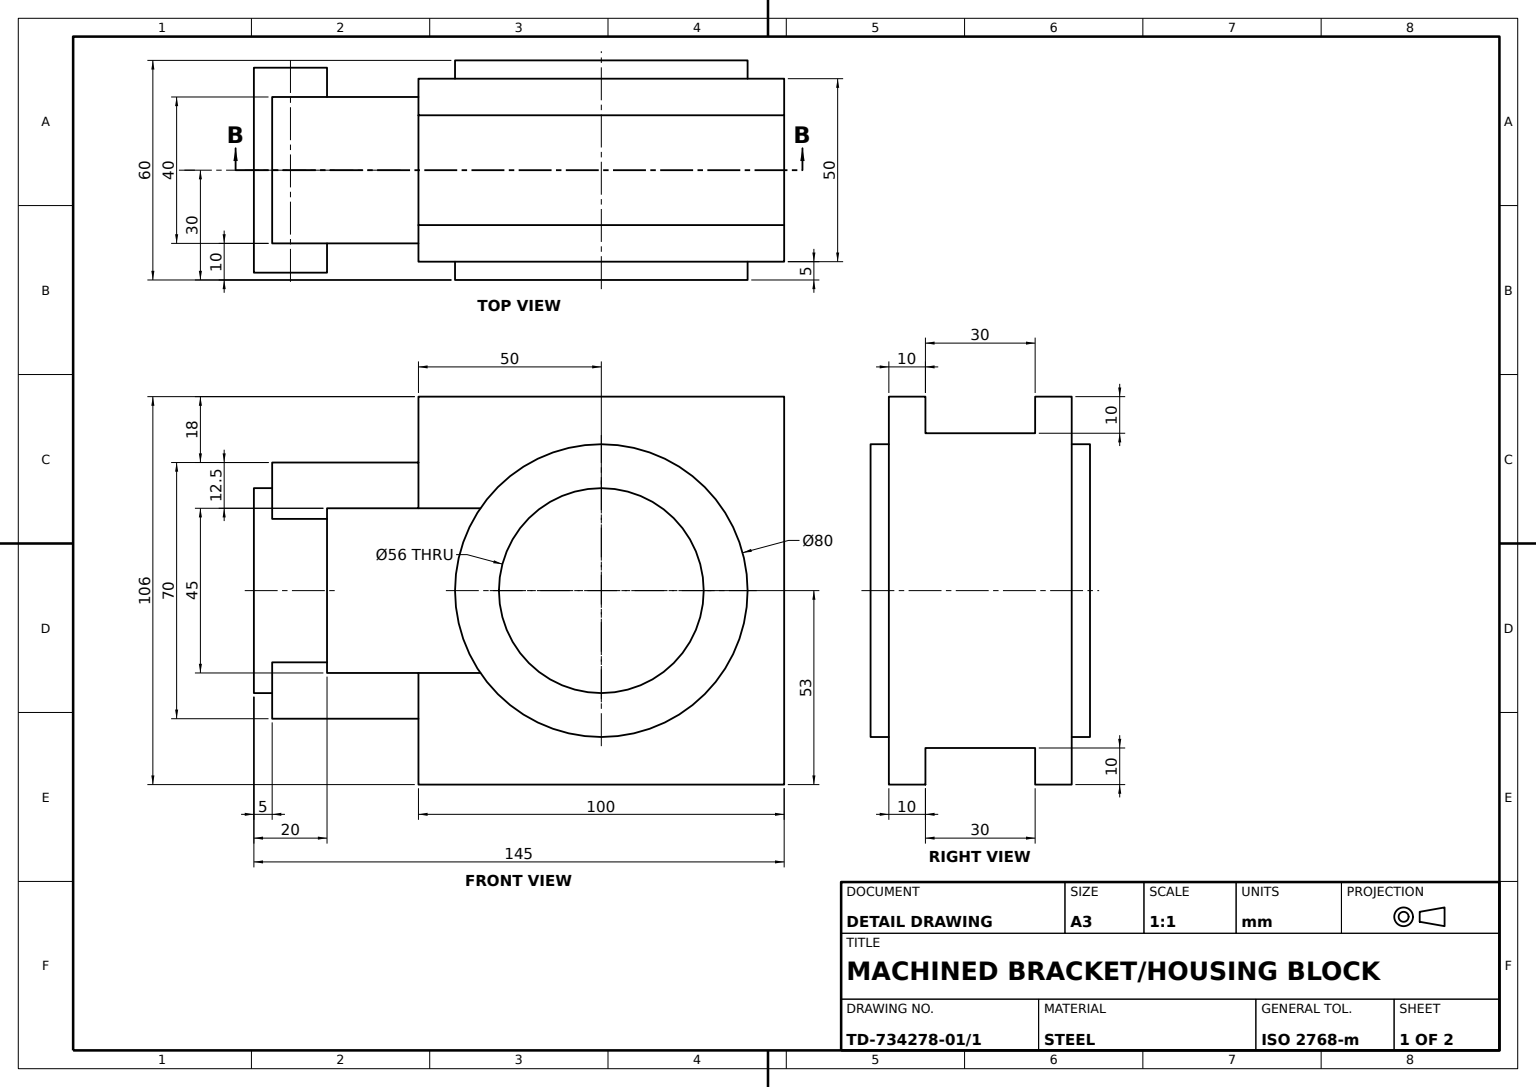
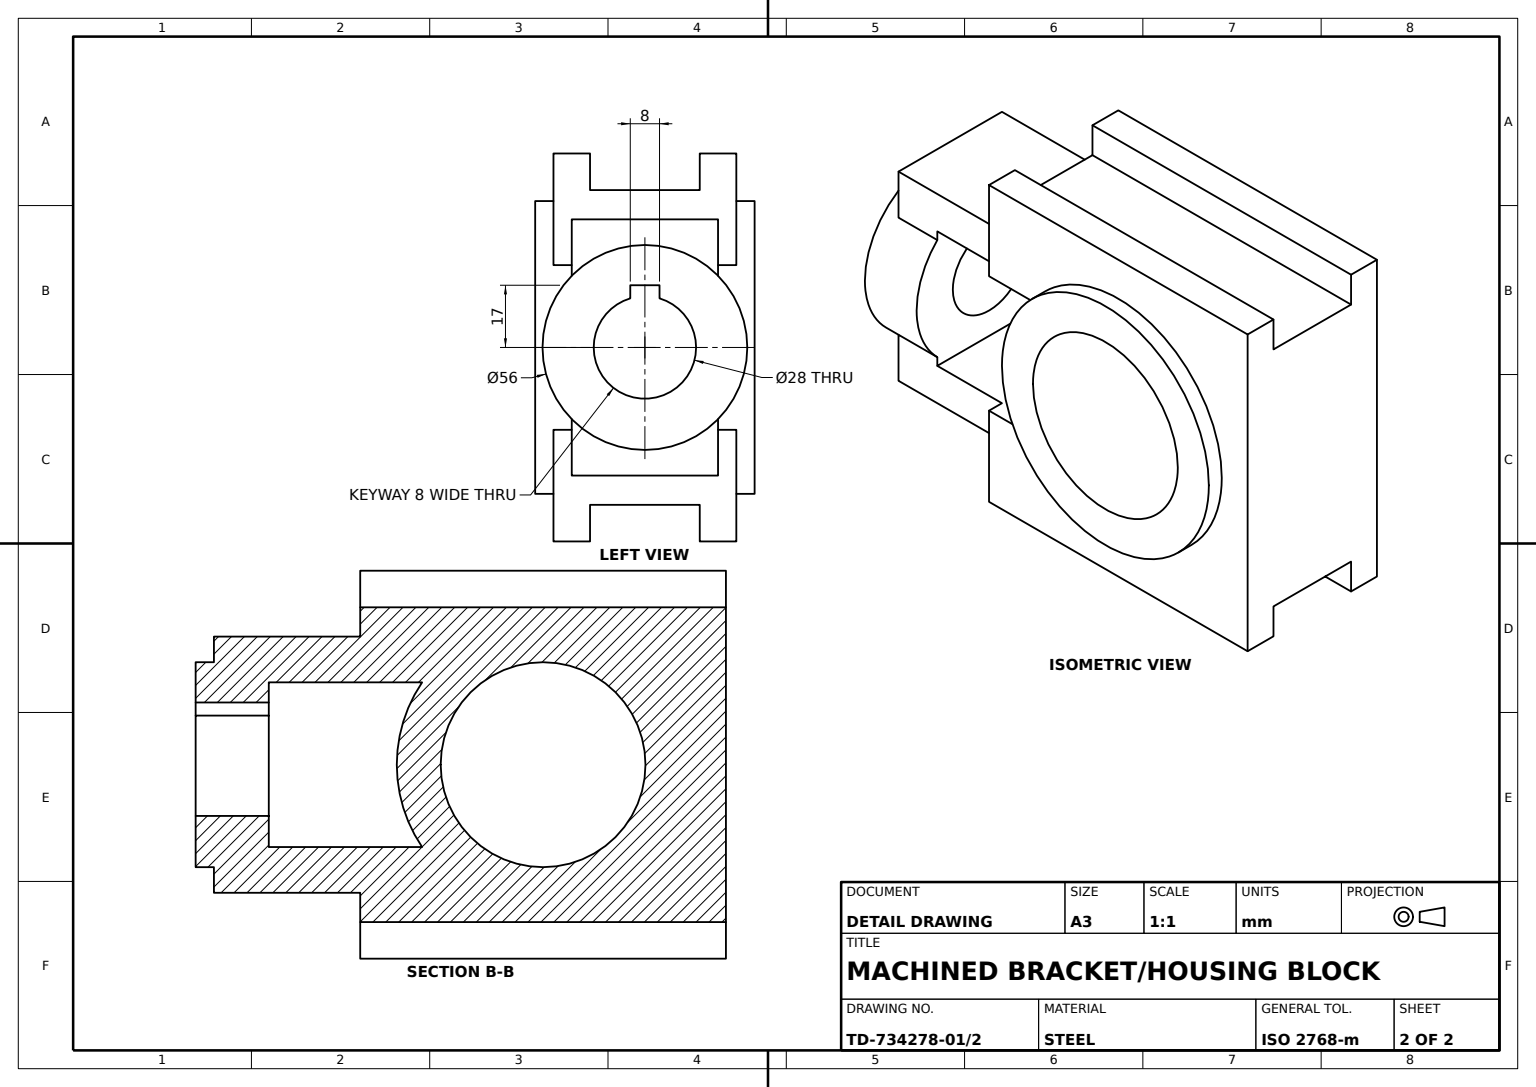
from build123d import *

# Parameters (mm, degrees)
BASE_BLOCK_DEPTH          = 50
BODY_RECESS_CUT_DEPTH     = 50
BEARING_HUB_PROFILE_R     = 40
BEARING_HUB_BOSS_DEPTH    = 50
HUB_START                 = 5
HUB_FLANGE_PROFILE_R      = 40
HUB_FLANGE_BOSS_DEPTH     = 5
MAIN_BORE_PROFILE_R       = 28
MAIN_BORE_CUT_DEPTH       = 113
TOP_SLOT_PROFILE_W        = 30
TOP_SLOT_PROFILE_H        = 100
TOP_SLOT_CUT_DEPTH        = 10
SIDE_ARM_BOSS_DEPTH       = 40
ARM_HOLE_PROFILE_R        = 28
ARM_HOLE_CUT_DEPTH        = 15
SHAFT_HUB_BOSS_DEPTH      = 5
SHAFT_HUB_BOSS_DEPTH_BACK = 15
SHAFT_HUB_PROFILE_R       = 28
KEYED_BORE_CUT_DEPTH      = 30
REAR_RING_PROFILE_R       = 40
REAR_RING_BOSS_DEPTH      = 5
THROUGH_BORE_PROFILE_R    = 28
THROUGH_BORE_CUT_DEPTH    = 194
SECOND_SLOT_PROFILE_W     = 30
SECOND_SLOT_PROFILE_H     = 100
SECOND_SLOT_CUT_DEPTH     = 10


with BuildPart() as part:
    # Base Block Profile → Base Block (new body)
    with BuildSketch(Plane(origin=(0, 0, 0), x_dir=(0, 0, -1), z_dir=(1, 0, 0))):
        Polygon((50, 0), (50, 53), (-50, 53), (-50, -53), (50, -53), align=None)
    extrude(amount=-BASE_BLOCK_DEPTH)

    # Body Recess Profile → Body Recess Cut (cut)
    with BuildSketch(Plane(origin=(0, 0, 0), x_dir=(0, 0, -1), z_dir=(1, 0, 0))):
        with BuildLine():
            Line((-50, 0), (-50, 22.5))
            Line((-50, 22.5), (-33.071891388, 22.5))
            ThreePointArc((-33.071891388, 22.5), (40, 0), (-33.071891388, -22.5))
            Line((-33.071891388, -22.5), (-50, -22.5))
            Line((-50, -22.5), (-50, 0))
        make_face()
    extrude(amount=-BODY_RECESS_CUT_DEPTH, mode=Mode.SUBTRACT)

    # Bearing Hub Profile → Bearing Hub Boss (add)
    with BuildSketch(Plane(origin=(0, 0, 0), x_dir=(0, 0, -1), z_dir=(1, 0, 0))):
        Circle(BEARING_HUB_PROFILE_R)
    extrude(amount=-BEARING_HUB_BOSS_DEPTH)

    # Hub Flange Profile → Hub Flange Boss (add)
    with BuildSketch(Plane(origin=(0, 0, 0), x_dir=(0, 0, -1), z_dir=(1, 0, 0)).offset(HUB_START)):
        Circle(HUB_FLANGE_PROFILE_R)
    extrude(amount=-HUB_FLANGE_BOSS_DEPTH)

    # Main Bore Profile → Main Bore Cut (cut)
    with BuildSketch(Plane(origin=(5, 0, 0), x_dir=(0, 0, -1), z_dir=(1, 0, 0))):
        Circle(MAIN_BORE_PROFILE_R)
    extrude(amount=-MAIN_BORE_CUT_DEPTH, mode=Mode.SUBTRACT)

    # Top Slot Profile → Top Slot Cut (cut)
    with BuildSketch(Plane(origin=(0, 53, 0), x_dir=(1, 0, 0), z_dir=(0, 1, 0))):
        with Locations((-25, 0)):
            Rectangle(TOP_SLOT_PROFILE_W, TOP_SLOT_PROFILE_H)
    extrude(amount=-TOP_SLOT_CUT_DEPTH, mode=Mode.SUBTRACT)

    # Side Arm Profile → Side Arm Boss (add)
    with BuildSketch(Plane(origin=(-5, 0, 0), x_dir=(0, 0, -1), z_dir=(1, 0, 0))):
        Polygon((-90, 0), (-90, 35), (-50, 35), (-50, 22.5), (-75, 22.5), (-75, -22.5), (-50, -22.5), (-50, -35), (-90, -35), align=None)
    extrude(amount=-SIDE_ARM_BOSS_DEPTH)

    # Arm Hole Profile → Arm Hole Cut (cut)
    with BuildSketch(Plane.XY.offset(90)):
        with Locations((-25, 0)):
            Circle(ARM_HOLE_PROFILE_R)
    extrude(amount=-ARM_HOLE_CUT_DEPTH, mode=Mode.SUBTRACT)

    # Shaft Hub Profile → Shaft Hub Boss (add, two sides: drawn at the far end of the back side and taken through both)
    with BuildSketch(Plane.XY.offset(90).offset(-SHAFT_HUB_BOSS_DEPTH_BACK)):
        with Locations((-25, 0)):
            Circle(SHAFT_HUB_PROFILE_R)
    extrude(amount=SHAFT_HUB_BOSS_DEPTH + SHAFT_HUB_BOSS_DEPTH_BACK)

    # Keyed Bore Profile → Keyed Bore Cut (cut)
    with BuildSketch(Plane.XY.offset(95)):
        with BuildLine():
            Line((-21, 13.416407865), (-21, 17))
            Line((-21, 17), (-29, 17))
            Line((-29, 17), (-29, 13.416407865))
            ThreePointArc((-29, 13.416407865), (-25, -14), (-21, 13.416407865))
        make_face()
    extrude(amount=-KEYED_BORE_CUT_DEPTH, mode=Mode.SUBTRACT)

    # Rear Ring Profile → Rear Ring Boss (add)
    with BuildSketch(Plane.ZY.offset(50)):
        with Locations(Location((0, 0, 0), (0, 0, 180))):
            Circle(REAR_RING_PROFILE_R)
    extrude(amount=REAR_RING_BOSS_DEPTH)

    # Through Bore Profile → Through Bore Cut (cut)
    with BuildSketch(Plane(origin=(5, 0, 0), x_dir=(0, 0, -1), z_dir=(1, 0, 0))):
        Circle(THROUGH_BORE_PROFILE_R)
    extrude(amount=-THROUGH_BORE_CUT_DEPTH, mode=Mode.SUBTRACT)

    # Second Slot Profile → Second Slot Cut (cut)
    with BuildSketch(Plane.XZ.offset(53)):
        with Locations((-25, 0)):
            Rectangle(SECOND_SLOT_PROFILE_W, SECOND_SLOT_PROFILE_H)
    extrude(amount=-SECOND_SLOT_CUT_DEPTH, mode=Mode.SUBTRACT)


solid = part.part
